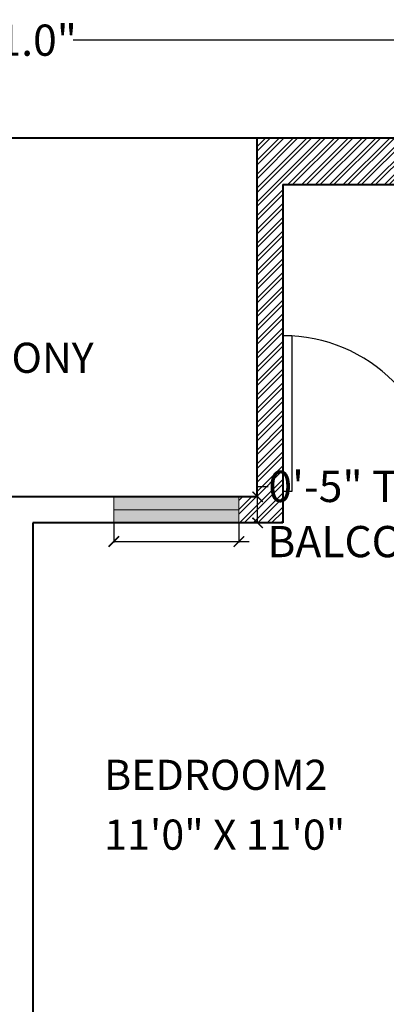
# Model space of a CAD drawing. Units: inches. Extents: x 528 to 2520, y -151 to 1354.
# Tile 22 of 41: x 1279 to 1350, y 1151 to 1340. Entities that reach past the tile are written whole.
import ezdxf

# ---------------------------------------------------------------- set-up
doc = ezdxf.new("R2010")
doc.units = ezdxf.units.IN
doc.header["$MEASUREMENT"] = 0
for name, color, linetype, lineweight in [('A-ANNO-DIMS', 2, 'Continuous', 18), ('A-AREA-IDEN', 7, 'Continuous', 18), ('A-Door', 150, 'Continuous', 25), ('A-WALL-PATT', 6, 'Continuous', 13), ('walls', 7, 'Continuous', 40), ('WINDOWS', 2, 'Continuous', 20)]:
    doc.layers.add(name, color=color, linetype=linetype, lineweight=lineweight)
doc.layers.add('A-GLAZ-PATT', color=152, linetype='Continuous', lineweight=13, true_color=0x2776bb)
doc.styles.get("Standard").update_dxf_attribs({"font": 'arial.ttf'})
doc.dimstyles.get("Standard").update_dxf_attribs({"dimtxt": 6, "dimasz": 2, "dimexe": 0.18, "dimexo": 0.0625, "dimgap": 0.09, "dimtad": 0, "dimtih": 1, "dimtoh": 1, "dimdec": 1, "dimzin": 0, "dimdsep": 46, "dimlunit": 3, "dimtxsty": 'Standard', "dimblk": 'ARCHTICK', "dimcen": 0.09, "dimadec": 0, "dimazin": 0, "dimtfac": 1, "dimtdec": 1, "dimtofl": 0, "dimtmove": 0, "dimatfit": 3, "dimfxl": 1, "dimtolj": 1, "dimtzin": 0, "dimarcsym": 0})

# ---------------------------------------------------------------- blocks, each defined once
blk = doc.blocks.new('_ArchTick')
at = {"color": 0, "linetype": 'ByBlock', "const_width": 0.15}
blk.add_lwpolyline([(-0.5, -0.5), (0.5, 0.5)], dxfattribs=at)
blk = doc.blocks.new('*D27')
at = {"layer": 'A-ANNO-DIMS', "color": 0, "lineweight": -2, "transparency": 16777216}
for p, q in [((1123.88, 1317.17), (1123.88, 1336.05)), ((1422.88, 1317.17), (1422.88, 1336.05)), ((1123.88, 1335.87), (1257.11, 1335.87)), ((1422.88, 1335.87), (1289.66, 1335.87))]:
    blk.add_line(p, q, dxfattribs=at)
at = {"layer": 'Defpoints', "color": 0, "transparency": 16777216}
for p in [(1422.88, 1335.87), (1123.88, 1317.1), (1422.88, 1317.1)]:
    blk.add_point(p, dxfattribs=at)
at = {"layer": 'A-ANNO-DIMS', "color": 0, "lineweight": -2, "transparency": 16777216, "xscale": 2, "yscale": 2, "zscale": 2, "rotation": 180}
blk.add_blockref('_ArchTick', (1123.88, 1335.87), dxfattribs=at)
at = {"layer": 'A-ANNO-DIMS', "color": 0, "lineweight": -2, "transparency": 16777216, "xscale": 2, "yscale": 2, "zscale": 2}
blk.add_blockref('_ArchTick', (1422.88, 1335.87), dxfattribs=at)
at = {"layer": 'A-ANNO-DIMS', "color": 0, "transparency": 16777216, "insert": (1273.38, 1335.87), "char_height": 6, "attachment_point": 5}
blk.add_mtext('\\A1;24\'-11.0"', dxfattribs=at)
blk = doc.blocks.new('DOOR-SWING-30')
for p, q in [((0, 6), (0, 0)), ((30, 6), (30, 0))]:
    blk.add_line(p, q)
blk.add_lwpolyline([(0, 6), (0, 36), (1.75, 36), (1.75, 6)], close=True)
blk.add_arc((0, 6), 30, 0, 90)
blk = doc.blocks.new('WINDOW-24x5-PLAN')
for p, q in [((0, 5), (24, 5)), ((24, 0), (24, 5)), ((0, 2.5), (24, 2.5))]:
    blk.add_line(p, q)
blk.add_lwpolyline([(0, 5), (24, 5), (24, 0), (0, 0)], close=True)
blk = doc.blocks.new('*D86')
at = {"layer": 'A-ANNO-DIMS', "color": 0, "lineweight": -2, "transparency": 16777216}
for p, q in [((1297.45, 1243.04), (1297.45, 1239.32)), ((1321.45, 1243.04), (1321.45, 1239.32)), ((1297.45, 1239.5), (1321.45, 1239.5)), ((1321.45, 1239.5), (1323.45, 1239.5))]:
    blk.add_line(p, q, dxfattribs=at)
at = {"layer": 'Defpoints', "color": 0, "transparency": 16777216}
for p in [(1297.45, 1243.1), (1321.45, 1243.1), (1321.45, 1239.5)]:
    blk.add_point(p, dxfattribs=at)
at = {"layer": 'A-ANNO-DIMS', "color": 0, "lineweight": -2, "transparency": 16777216, "xscale": 2, "yscale": 2, "zscale": 2, "rotation": 180}
blk.add_blockref('_ArchTick', (1297.45, 1239.5), dxfattribs=at)
at = {"layer": 'A-ANNO-DIMS', "color": 0, "lineweight": -2, "transparency": 16777216, "xscale": 2, "yscale": 2, "zscale": 2}
blk.add_blockref('_ArchTick', (1321.45, 1239.5), dxfattribs=at)
at = {"layer": 'A-ANNO-DIMS', "color": 0, "transparency": 16777216, "insert": (1382.44, 1239.5), "char_height": 6, "attachment_point": 5}
blk.add_mtext('\\A1;BALCONY WINDOW 2\'-0" TYP.', dxfattribs=at)
blk = doc.blocks.new('*D87')
at = {"layer": 'A-ANNO-DIMS', "color": 0, "lineweight": -2, "transparency": 16777216}
for p, q in [((1325.05, 1248.1), (1325.05, 1250.1)), ((1325.05, 1250.1), (1327.05, 1250.1)), ((1321.51, 1248.1), (1325.23, 1248.1)), ((1325.05, 1243.1), (1325.05, 1248.1)), ((1321.51, 1243.1), (1325.23, 1243.1))]:
    blk.add_line(p, q, dxfattribs=at)
at = {"layer": 'Defpoints', "color": 0, "transparency": 16777216}
for p in [(1321.45, 1248.1), (1325.05, 1248.1), (1321.45, 1243.1)]:
    blk.add_point(p, dxfattribs=at)
at = {"layer": 'A-ANNO-DIMS', "color": 0, "lineweight": -2, "transparency": 16777216, "xscale": 2, "yscale": 2, "zscale": 2}
for p, rotation in [((1325.05, 1248.1), 90), ((1325.05, 1243.1), 270)]:
    blk.add_blockref('_ArchTick', p, dxfattribs=dict(at, rotation=rotation))
at = {"layer": 'A-ANNO-DIMS', "color": 0, "transparency": 16777216, "insert": (1345.43, 1250.1), "char_height": 6, "attachment_point": 5}
blk.add_mtext('\\A1;0\'-5" TYP.', dxfattribs=at)

msp = doc.modelspace()

# ---------------------------------------------------------------- hatches: boundary and pattern name
at = {"layer": 'A-GLAZ-PATT'}
h = msp.add_hatch(color=256, dxfattribs=at)
h.dxf.hatch_style = 1
h.paths.add_polyline_path([(1321.45, 1248.1), (1297.45, 1248.1), (1297.45, 1245.6), (1321.45, 1245.6)])
h.paths.add_polyline_path([(1321.45, 1245.6), (1297.45, 1245.6), (1297.45, 1243.1), (1321.45, 1243.1)])
at = {"layer": 'A-WALL-PATT'}
h = msp.add_hatch(dxfattribs=at)
h.set_pattern_fill('ANSI32', color=256, scale=5)
h.set_pattern_definition([(45, (537.1868, 0), (-1.3258252, 1.3258252), []), (45, (538.0707, 0), (-1.3258252, 1.3258252), [])])
h.paths.add_polyline_path([(1132.88, 1163.86), (1123.88, 1163.86), (1123.88, 969.1), (1135.43, 969.1), (1140.43, 969.1), (1140.43, 974.1), (1132.88, 974.1), (1132.88, 1082.1), (1228.88, 1082.1), (1228.88, 1087.1), (1228.88, 1106.1), (1234.88, 1106.1), (1234.88, 1111.1), (1223.88, 1111.1), (1223.88, 1087.1), (1132.88, 1087.1)])
h.paths.add_polyline_path([(1225.89, 974.1), (1188.43, 974.1), (1188.43, 969.1), (1225.89, 969.1)])
h.paths.add_polyline_path([(1422.88, 1171.37), (1413.88, 1171.37), (1413.88, 1111.1), (1323.88, 1111.1), (1323.88, 1106.1), (1413.88, 1106.1), (1413.88, 974.1), (1323.88, 974.1), (1323.88, 969.1), (1413.88, 969.1), (1413.88, 825.1), (1371.88, 825.1), (1371.88, 816.1), (1422.88, 816.1)])
h.paths.add_polyline_path([(1422.88, 1317.1), (1413.84, 1317.1), (1413.84, 1308.1), (1413.88, 1308.1), (1413.88, 1248.1), (1359.88, 1248.1), (1359.88, 1243.1), (1413.88, 1243.1), (1413.88, 1219.37), (1422.88, 1219.37)])
h.paths.add_polyline_path([(1389.84, 1317.1), (1324.88, 1317.1), (1324.88, 1248.1), (1321.45, 1248.1), (1321.45, 1243.1), (1329.88, 1243.1), (1329.88, 1249.1), (1329.88, 1308.1), (1389.84, 1308.1)])
h.paths.add_polyline_path([(1221.88, 1317.1), (1156.88, 1317.1), (1156.88, 1308.1), (1216.88, 1308.1), (1216.88, 1248.1), (1216.88, 1243.1), (1221.88, 1243.1), (1221.88, 1248.25)])
h.paths.add_polyline_path([(1132.88, 1308.1), (1132.88, 1317.1), (1123.88, 1317.1), (1123.88, 1211.86), (1132.88, 1211.86), (1132.88, 1243.1), (1186.88, 1243.1), (1186.88, 1248.1), (1132.88, 1248.1)])
h.paths.add_polyline_path([(1281.88, 969.1), (1281.88, 974.1), (1261.89, 974.1), (1261.89, 969.1), (1276.88, 969.1), (1276.88, 874.29), (1281.88, 874.29)])
h.paths.add_polyline_path([(1276.88, 969.1), (1264.88, 969.1), (1264.88, 965.12), (1267.92, 965.12), (1267.92, 961.68), (1271.62, 961.68), (1271.62, 957.24), (1276.88, 957.24)], flags=17)
h.paths.add_polyline_path([(1323.88, 825.1), (1281.88, 825.1), (1281.88, 832.29), (1276.88, 832.29), (1276.88, 816.1), (1323.88, 816.1)])

# ---------------------------------------------------------------- linework, layer by layer
at = {"layer": 'walls'}
for p, q in [((1221.88, 1317.1), (1324.88, 1317.1)), ((1324.88, 1317.1), (1324.88, 1248.1)), ((1324.88, 1317.1), (1422.88, 1317.1)), ((1329.88, 1308.1), (1329.88, 1248.1)), ((1329.88, 1308.1), (1413.88, 1308.1)), ((1324.88, 1248.1), (1257.88, 1248.1)), ((1329.88, 1248.1), (1329.88, 1243.1)), ((1281.88, 1243.1), (1281.88, 1111.1)), ((1329.88, 1243.1), (1281.88, 1243.1))]:
    msp.add_line(p, q, dxfattribs=at)

# ---------------------------------------------------------------- block references
at = {"layer": 'A-Door'}
msp.add_blockref('DOOR-SWING-30', (1329.88, 1243.1), dxfattribs=at)
at = {"layer": 'WINDOWS'}
msp.add_blockref('WINDOW-24x5-PLAN', (1297.45, 1243.1), dxfattribs=at)

# ---------------------------------------------------------------- texts
at = {"layer": 'A-AREA-IDEN'}
for s, height, p in [('BALCONY', 5.793, (1258.47, 1271.93)), ('BEDROOM2', 5.793, (1295.6, 1191.78)), ('11\'0" X 11\'0"', 5.7926, (1295.6, 1180.28))]:
    msp.add_text(s, height=height, dxfattribs=at).set_placement(p)

# ---------------------------------------------------------------- dimensions: what is measured, and where the dimension line sits
at = {"layer": 'A-ANNO-DIMS'}
dim = msp.add_linear_dim(base=(1422.88, 1335.87), p1=(1123.88, 1317.1), p2=(1422.88, 1317.1), dimstyle='Standard', override={"dimclrd": 0, "dimclre": 0, "dimclrt": 0}, dxfattribs=at)
dim.commit()
dim.dimension.update_dxf_attribs({"geometry": '*D27', "text_midpoint": (1273.38, 1335.87)})
dim = msp.add_linear_dim(base=(1321.45, 1239.5), p1=(1297.45, 1243.1), p2=(1321.45, 1243.1), text='BALCONY WINDOW <> TYP.', dimstyle='Standard', override={"dimdec": 1, "dimlfac": 1, "dimrnd": 0, "dimzin": 1, "dimdsep": 46, "dimlunit": 4, "dimfrac": 2}, dxfattribs=at)
dim.commit()
dim.dimension.update_dxf_attribs({"geometry": '*D86', "text_midpoint": (1382.44, 1239.5)})
dim = msp.add_linear_dim(base=(1325.05, 1248.1), p1=(1321.45, 1243.1), p2=(1321.45, 1248.1), angle=90, text='<> TYP.', dimstyle='Standard', override={"dimdec": 1, "dimlfac": 1, "dimrnd": 0, "dimzin": 1, "dimdsep": 46, "dimlunit": 4, "dimfrac": 2}, dxfattribs=at)
dim.commit()
dim.dimension.update_dxf_attribs({"geometry": '*D87', "text_midpoint": (1345.43, 1250.1)})

doc.saveas('drawing.dxf')
